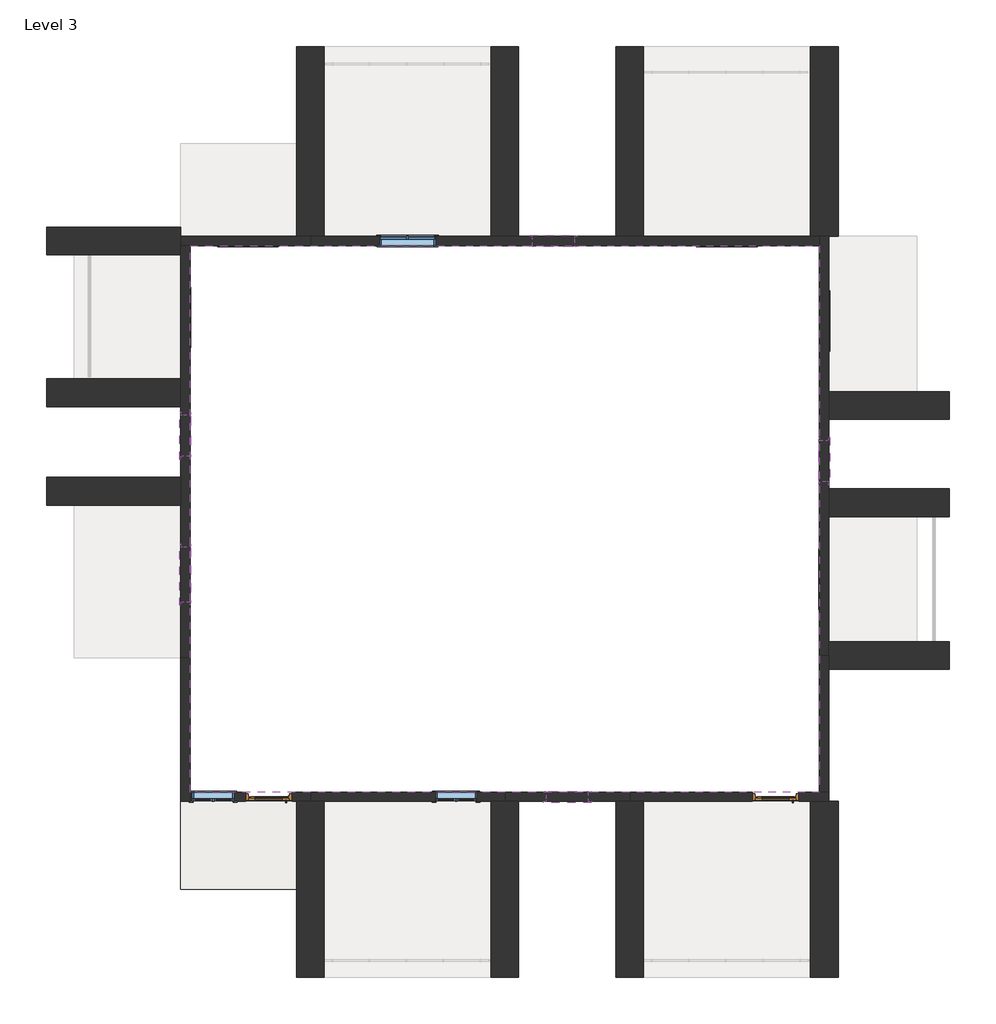
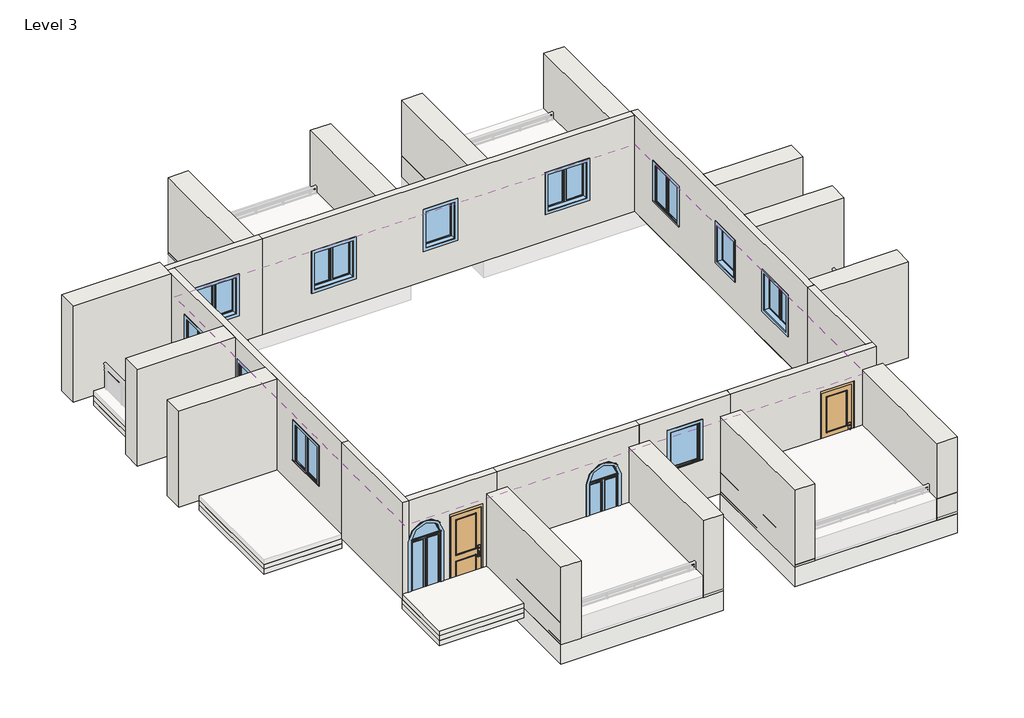
# One storey, part 1 of 2: 24 walls, 13 windows, 5 slabs, 2 doors, 1 covering.
"""IFC4 building model written with IfcOpenShell, lengths in millimetres."""

from ifc_helpers import new_model, si_unit, frame, origin, place, context, project, spatial, polyline, circle_curve, outline, extrude, faceted_brep, transform, mapped, element, save
from ifc_brep_helpers import plane_surface, revolved_surface, advanced_brep
from components import door_b6c2ee01, window_4e95f2a8, window_0862ab64, window_3a1167bf, window_8a4441b2

model = new_model("IFC4")

# Units and contexts
model_context = context("Model", 3, world=origin())
ifc_project = project(units=[si_unit("LENGTHUNIT", "METRE", prefix="MILLI")], contexts=[model_context])

# Site, building, storey
site = spatial("IfcSite", under=ifc_project)
building = spatial("IfcBuilding", under=site)
storey = spatial("IfcBuildingStorey", under=building, Name="Level 3", Elevation=6096.0)

# Covering
placement = place(None, origin())
element("IfcCovering", 1, ObjectType="2' x 4' ACT System", at=placement, inside=storey, context=model_context, shape_type="SweptSolid", body=[
    extrude(outline(polyline([(-12179.4937431, 6319.013611), (-9537.8937431, 6319.013611), (1638.1062569, 6319.013611), (1638.1062569, -2672.586389), (1638.1062569, -5669.786389), (-2527.4937431, -5669.786389), (-5270.6937431, -5669.786389), (-9537.8937431, -5669.786389), (-12179.4937431, -5669.786389), (-12179.4937431, -2723.386389), (-12179.4937431, 6319.013611)])), frame((0.0, 0.0, 8534.4), z_axis=(0.0, 0.0, 1.0), x_axis=(1.0, 0.0, 0.0)), (0.0, 0.0, 1.0), 57.15),
])

# Doors
door_shape = door_b6c2ee01(model_context)
element("IfcDoor", 2, ObjectType="Door-Exterior-Single-Two_Lite : 36\" x 94\"", at=placement, inside=storey, context=model_context, shape_type="MappedRepresentation", body=[
    mapped(door_shape, transform((-10452.2937431, -5765.036389, 6096.0), x_axis=(-1.0, 0.0, 0.0), y_axis=(0.0, -1.0, 0.0), z_axis=(0.0, 0.0, 1.0))),
])
element("IfcDoor", 3, ObjectType="Door-Exterior-Single-Two_Lite : 36\" x 94\"", at=placement, inside=storey, context=model_context, shape_type="MappedRepresentation", body=[
    mapped(door_shape, transform((672.9062569, -5765.036389, 6096.0), x_axis=(-1.0, 0.0, 0.0), y_axis=(0.0, -1.0, 0.0), z_axis=(0.0, 0.0, 1.0))),
])

# Slabs
element("IfcSlab", 4, ObjectType="Generic - 2' 2", at=placement, inside=storey, context=model_context, shape_type="SweptSolid", body=[
    extrude(outline(polyline([(-4965.8937431, -9733.786389), (-9842.6937431, -9733.786389), (-9842.6937431, -5872.986389), (-4965.8937431, -5872.986389), (-4965.8937431, -9733.786389)])), frame((0.0, 0.0, 5791.2), z_axis=(0.0, 0.0, 1.0), x_axis=(1.0, 0.0, 0.0)), (0.0, 0.0, 1.0), 609.6),
])
element("IfcSlab", 5, ObjectType="Generic - 2' 2", at=placement, inside=storey, context=model_context, shape_type="SweptSolid", body=[
    extrude(outline(polyline([(2044.5062569, -9733.786389), (-2832.2937431, -9733.786389), (-2832.2937431, -5872.986389), (2044.5062569, -5872.986389), (2044.5062569, -9733.786389)])), frame((0.0, 0.0, 5791.2), z_axis=(0.0, 0.0, 1.0), x_axis=(1.0, 0.0, 0.0)), (0.0, 0.0, 1.0), 609.6),
])
element("IfcSlab", 6, ObjectType="general 6\"", at=placement, inside=storey, context=model_context, shape_type="SweptSolid", body=[
    extrude(outline(polyline([(-14722.8064179, 6115.813611), (-12382.6937431, 6115.813611), (-12382.6937431, 3398.013611), (-14722.8064179, 3398.013611), (-14722.8064179, 6115.813611)])), frame((0.0, 0.0, 6096.0), z_axis=(0.0, 0.0, 1.0), x_axis=(1.0, 0.0, 0.0)), (0.0, 0.0, 1.0), 152.4),
    extrude(outline(polyline([(-14722.8064179, 629.413611), (-12382.6937431, 629.413611), (-12382.6937431, -2723.386389), (-14722.8064179, -2723.386389), (-14722.8064179, 629.413611)])), frame((0.0, 0.0, 6096.0), z_axis=(0.0, 0.0, 1.0), x_axis=(1.0, 0.0, 0.0)), (0.0, 0.0, 1.0), 152.4),
    extrude(outline(polyline([(-9842.6937431, -5872.986389), (-9842.6937431, -7803.386389), (-12382.6937431, -7803.386389), (-12382.6937431, -5872.986389), (-9842.6937431, -5872.986389)])), frame((0.0, 0.0, 6096.0), z_axis=(0.0, 0.0, 1.0), x_axis=(1.0, 0.0, 0.0)), (0.0, 0.0, 1.0), 152.4),
    extrude(outline(polyline([(3771.7062569, -2367.786389), (1841.3062569, -2367.786389), (1841.3062569, 426.213611), (3771.7062569, 426.213611), (3771.7062569, -2367.786389)])), frame((0.0, 0.0, 6096.0), z_axis=(0.0, 0.0, 1.0), x_axis=(1.0, 0.0, 0.0)), (0.0, 0.0, 1.0), 152.4),
    extrude(outline(polyline([(3771.7062569, 3118.613611), (1841.3062569, 3118.613611), (1841.3062569, 6522.213611), (3771.7062569, 6522.213611), (3771.7062569, 3118.613611)])), frame((0.0, 0.0, 6096.0), z_axis=(0.0, 0.0, 1.0), x_axis=(1.0, 0.0, 0.0)), (0.0, 0.0, 1.0), 152.4),
    extrude(outline(polyline([(-12382.6937431, 6522.213611), (-12382.6937431, 8557.6995084), (-9842.6937431, 8557.6995084), (-9842.6937431, 6522.213611), (-12382.6937431, 6522.213611)])), frame((0.0, 0.0, 6096.0), z_axis=(0.0, 0.0, 1.0), x_axis=(1.0, 0.0, 0.0)), (0.0, 0.0, 1.0), 152.4),
])
element("IfcSlab", 7, ObjectType="general 6\" 2", at=placement, inside=storey, context=model_context, shape_type="SweptSolid", body=[
    extrude(outline(polyline([(3771.7062569, -2367.786389), (1841.3062569, -2367.786389), (1841.3062569, 375.413611), (3771.7062569, 375.413611), (3771.7062569, -2367.786389)])), frame((0.0, 0.0, 6248.4), z_axis=(0.0, 0.0, 1.0), x_axis=(1.0, 0.0, 0.0)), (0.0, 0.0, 1.0), 152.4),
    extrude(outline(polyline([(3771.7062569, 3118.613611), (1841.3062569, 3118.613611), (1841.3062569, 6522.213611), (3771.7062569, 6522.213611), (3771.7062569, 3118.613611)])), frame((0.0, 0.0, 6248.4), z_axis=(0.0, 0.0, 1.0), x_axis=(1.0, 0.0, 0.0)), (0.0, 0.0, 1.0), 152.4),
    extrude(outline(polyline([(-12382.6937431, 6522.213611), (-12382.6937431, 8557.6995084), (-9842.6937431, 8557.6995084), (-9842.6937431, 6522.213611), (-12382.6937431, 6522.213611)])), frame((0.0, 0.0, 6248.4), z_axis=(0.0, 0.0, 1.0), x_axis=(1.0, 0.0, 0.0)), (0.0, 0.0, 1.0), 152.4),
    extrude(outline(polyline([(-14722.8064179, 6115.813611), (-12384.3500805, 6115.813611), (-12384.3500805, 3398.013611), (-14722.8064179, 3398.013611), (-14722.8064179, 6115.813611)])), frame((0.0, 0.0, 6248.4), z_axis=(0.0, 0.0, 1.0), x_axis=(1.0, 0.0, 0.0)), (0.0, 0.0, 1.0), 152.4),
    extrude(outline(polyline([(-14722.8064179, -2723.386389), (-14722.8064179, 629.413611), (-12382.6937431, 629.413611), (-12382.6937431, -2723.386389), (-14722.8064179, -2723.386389)])), frame((0.0, 0.0, 6248.4), z_axis=(0.0, 0.0, 1.0), x_axis=(1.0, 0.0, 0.0)), (0.0, 0.0, 1.0), 152.4),
    extrude(outline(polyline([(-9842.6937431, -5872.986389), (-9842.6937431, -7803.386389), (-12382.6937431, -7803.386389), (-12382.6937431, -5872.986389), (-9842.6937431, -5872.986389)])), frame((0.0, 0.0, 6248.4), z_axis=(0.0, 0.0, 1.0), x_axis=(1.0, 0.0, 0.0)), (0.0, 0.0, 1.0), 152.4),
])
element("IfcSlab", 8, ObjectType="general 6\" 3", at=placement, inside=storey, context=model_context, shape_type="SweptSolid", body=[
    extrude(outline(polyline([(-12382.6937431, -5872.986389), (-9842.6937431, -5872.986389), (-9842.6937431, -7803.386389), (-12382.6937431, -7803.386389), (-12382.6937431, -5872.986389)])), frame((0.0, 0.0, 6400.8), z_axis=(0.0, 0.0, 1.0), x_axis=(1.0, 0.0, 0.0)), (0.0, 0.0, 1.0), 152.4),
])

# Walls
element("IfcWall", 9, ObjectType="Generic - 8\"", at=placement, inside=storey, context=model_context, shape_type="Brep", body=[
    faceted_brep([(-12382.6937431, 6319.013611, 6400.8), (-12179.4937431, 6319.013611, 6400.8), (-9537.8937431, 6319.013611, 6400.8), (-9537.8937431, 6319.013611, 9448.8), (-12179.4937431, 6319.013611, 9448.8), (-12382.6937431, 6319.013611, 9448.8), (-10299.8937431, 6319.013611, 8534.4), (-10299.8937431, 6319.013611, 7315.2), (-11519.0937431, 6319.013611, 7315.2), (-11519.0937431, 6319.013611, 8534.4), (-12382.6937431, 6522.213611, 6400.8), (-12382.6937431, 6522.213611, 9448.8), (-9537.8937431, 6522.213611, 9448.8), (-9537.8937431, 6522.213611, 6400.8), (-9842.6937431, 6522.213611, 6400.8), (-10299.8937431, 6522.213611, 8534.4), (-11519.0937431, 6522.213611, 8534.4), (-11519.0937431, 6522.213611, 7315.2), (-10299.8937431, 6522.213611, 7315.2)], [[[0, 1, 2, 3, 4, 5], [6, 7, 8, 9]], [[10, 11, 12, 13, 14], [15, 16, 17, 18]], [[2, 1, 0, 10, 14, 13]], [[5, 4, 3, 12, 11]], [[0, 5, 11, 10]], [[7, 6, 15, 18]], [[8, 7, 18, 17]], [[9, 8, 17, 16]], [[6, 9, 16, 15]], [[2, 13, 12, 3]]]),
])
element("IfcWall", 10, ObjectType="Generic - 8\"", at=placement, inside=storey, context=model_context, shape_type="Brep", body=[
    faceted_brep([(-12179.4937431, -5872.986389, 6400.8), (-12179.4937431, -5669.786389, 6400.8), (-12179.4937431, -2723.386389, 6400.8), (-12179.4937431, -2723.386389, 9448.8), (-12179.4937431, -5669.786389, 9448.8), (-12179.4937431, -5872.986389, 9448.8), (-12382.6937431, -5872.986389, 6400.8), (-12382.6937431, -5872.986389, 9448.8), (-12382.6937431, -2723.386389, 9448.8), (-12382.6937431, -2723.386389, 6400.8)], [[[0, 1, 2, 3, 4, 5]], [[6, 7, 8, 9]], [[2, 1, 0, 6, 9]], [[3, 2, 9, 8]], [[5, 4, 3, 8, 7]], [[0, 5, 7, 6]]]),
])
element("IfcWall", 11, ObjectType="Generic - 8\"", at=placement, inside=storey, context=model_context, shape_type="Brep", body=[
    faceted_brep([(-2527.4937431, -5669.786389, 9448.8), (1638.1062569, -5669.786389, 9448.8), (1841.3062569, -5669.786389, 9448.8), (1841.3062569, -5669.786389, 6400.8), (1638.1062569, -5669.786389, 6400.8), (1180.9062569, -5669.786389, 6400.8), (1180.9062569, -5669.786389, 8585.2), (164.9062569, -5669.786389, 8585.2), (164.9062569, -5669.786389, 6400.8), (-2527.4937431, -5669.786389, 6400.8), (1841.3062569, -5872.986389, 9448.8), (-2527.4937431, -5872.986389, 9448.8), (-2527.4937431, -5872.986389, 6400.8), (-2222.6937431, -5872.986389, 6400.8), (164.9062569, -5872.986389, 6400.8), (164.9062569, -5872.986389, 8585.2), (1180.9062569, -5872.986389, 8585.2), (1180.9062569, -5872.986389, 6400.8), (1434.9062569, -5872.986389, 6400.8), (1841.3062569, -5872.986389, 6400.8)], [[[0, 1, 2, 3, 4, 5, 6, 7, 8, 9]], [[10, 11, 12, 13, 14, 15, 16, 17, 18, 19]], [[3, 19, 18, 17, 5, 4]], [[12, 9, 8, 14, 13]], [[2, 1, 0, 11, 10]], [[2, 10, 19, 3]], [[7, 15, 14, 8]], [[15, 7, 6, 16]], [[16, 6, 5, 17]], [[9, 12, 11, 0]]]),
])
element("IfcWall", 12, ObjectType="Generic - 8\"", at=placement, inside=storey, context=model_context, shape_type="Brep", body=[
    faceted_brep([(1638.1062569, 6522.213611, 9448.8), (1638.1062569, 6522.213611, 6400.8), (1638.1062569, 6319.013611, 6400.8), (1638.1062569, -2672.586389, 6400.8), (1638.1062569, -2672.586389, 9448.8), (1638.1062569, 6319.013611, 9448.8), (1638.1062569, 1137.413611, 8605.6747769), (1638.1062569, 1137.413611, 7386.4747769), (1638.1062569, 2051.813611, 7386.4747769), (1638.1062569, 2051.813611, 8605.6747769), (1638.1062569, -1605.786389, 8545.5712595), (1638.1062569, -1605.786389, 7326.3712595), (1638.1062569, -386.586389, 7326.3712595), (1638.1062569, -386.586389, 8545.5712595), (1638.1062569, 4058.413611, 8545.5712595), (1638.1062569, 4058.413611, 7326.3712595), (1638.1062569, 5277.613611, 7326.3712595), (1638.1062569, 5277.613611, 8545.5712595), (1841.3062569, 6522.213611, 6400.8), (1841.3062569, 6522.213611, 9448.8), (1841.3062569, 3118.613611, 9448.8), (1841.3062569, 2509.013611, 9448.8), (1841.3062569, 985.013611, 9448.8), (1841.3062569, 375.413611, 9448.8), (1841.3062569, -2367.786389, 9448.8), (1841.3062569, -2672.586389, 9448.8), (1841.3062569, -2672.586389, 6400.8), (1841.3062569, -2367.786389, 6400.8), (1841.3062569, 375.413611, 6400.8), (1841.3062569, 985.013611, 6400.8), (1841.3062569, 2509.013611, 6400.8), (1841.3062569, 3118.613611, 6400.8), (1841.3062569, 1137.413611, 8605.6747769), (1841.3062569, 2051.813611, 8605.6747769), (1841.3062569, 2051.813611, 7386.4747769), (1841.3062569, 1137.413611, 7386.4747769), (1841.3062569, -1605.786389, 8545.5712595), (1841.3062569, -386.586389, 8545.5712595), (1841.3062569, -386.586389, 7326.3712595), (1841.3062569, -1605.786389, 7326.3712595), (1841.3062569, 4058.413611, 8545.5712595), (1841.3062569, 5277.613611, 8545.5712595), (1841.3062569, 5277.613611, 7326.3712595), (1841.3062569, 4058.413611, 7326.3712595)], [[[0, 1, 2, 3, 4, 5], [6, 7, 8, 9], [10, 11, 12, 13], [14, 15, 16, 17]], [[18, 19, 20, 21, 22, 23, 24, 25, 26, 27, 28, 29, 30, 31], [32, 33, 34, 35], [36, 37, 38, 39], [40, 41, 42, 43]], [[3, 2, 1, 18, 31, 30, 29, 28, 27, 26]], [[4, 3, 26, 25]], [[0, 5, 4, 25, 24, 23, 22, 21, 20, 19]], [[0, 19, 18, 1]], [[7, 6, 32, 35]], [[8, 7, 35, 34]], [[9, 8, 34, 33]], [[6, 9, 33, 32]], [[11, 10, 36, 39]], [[12, 11, 39, 38]], [[13, 12, 38, 37]], [[10, 13, 37, 36]], [[15, 14, 40, 43]], [[16, 15, 43, 42]], [[17, 16, 42, 41]], [[14, 17, 41, 40]]]),
])
element("IfcWall", 13, ObjectType="Generic - 8\"", at=placement, inside=storey, context=model_context, shape_type="Brep", body=[
    faceted_brep([(-12179.4937431, -2723.386389, 6400.8), (-12179.4937431, 6319.013611, 6400.8), (-12179.4937431, 6319.013611, 9448.8), (-12179.4937431, -2723.386389, 9448.8), (-12179.4937431, 2610.613611, 8771.7149116), (-12179.4937431, 2610.613611, 7552.5149116), (-12179.4937431, 1696.213611, 7552.5149116), (-12179.4937431, 1696.213611, 8771.7149116), (-12179.4937431, -284.986389, 8594.8059909), (-12179.4937431, -284.986389, 7375.6059909), (-12179.4937431, -1504.186389, 7375.6059909), (-12179.4937431, -1504.186389, 8594.8059909), (-12179.4937431, 5353.813611, 8521.1335827), (-12179.4937431, 5353.813611, 7301.9335827), (-12179.4937431, 4134.613611, 7301.9335827), (-12179.4937431, 4134.613611, 8521.1335827), (-12382.6937431, -2723.386389, 6400.8), (-12382.6937431, -2723.386389, 9448.8), (-12382.6937431, 629.413611, 9448.8), (-12382.6937431, 1239.013611, 9448.8), (-12382.6937431, 2788.413611, 9448.8), (-12382.6937431, 3398.013611, 9448.8), (-12382.6937431, 6115.813611, 9448.8), (-12382.6937431, 6319.013611, 9448.8), (-12382.6937431, 6319.013611, 6400.8), (-12382.6937431, 6115.813611, 6400.8), (-12382.6937431, 3398.013611, 6400.8), (-12382.6937431, 2788.413611, 6400.8), (-12382.6937431, 1239.013611, 6400.8), (-12382.6937431, 629.413611, 6400.8), (-12382.6937431, 2610.613611, 8771.7149116), (-12382.6937431, 1696.213611, 8771.7149116), (-12382.6937431, 1696.213611, 7552.5149116), (-12382.6937431, 2610.613611, 7552.5149116), (-12382.6937431, -284.986389, 8594.8059909), (-12382.6937431, -1504.186389, 8594.8059909), (-12382.6937431, -1504.186389, 7375.6059909), (-12382.6937431, -284.986389, 7375.6059909), (-12382.6937431, 5353.813611, 8521.1335827), (-12382.6937431, 4134.613611, 8521.1335827), (-12382.6937431, 4134.613611, 7301.9335827), (-12382.6937431, 5353.813611, 7301.9335827)], [[[0, 1, 2, 3], [4, 5, 6, 7], [8, 9, 10, 11], [12, 13, 14, 15]], [[16, 17, 18, 19, 20, 21, 22, 23, 24, 25, 26, 27, 28, 29], [30, 31, 32, 33], [34, 35, 36, 37], [38, 39, 40, 41]], [[1, 0, 16, 29, 28, 27, 26, 25, 24]], [[3, 2, 23, 22, 21, 20, 19, 18, 17]], [[0, 3, 17, 16]], [[2, 1, 24, 23]], [[5, 4, 30, 33]], [[6, 5, 33, 32]], [[7, 6, 32, 31]], [[4, 7, 31, 30]], [[9, 8, 34, 37]], [[10, 9, 37, 36]], [[11, 10, 36, 35]], [[8, 11, 35, 34]], [[13, 12, 38, 41]], [[14, 13, 41, 40]], [[15, 14, 40, 39]], [[12, 15, 39, 38]]]),
])
element("IfcWall", 14, ObjectType="Generic - 8\"", at=placement, inside=storey, context=model_context, shape_type="AdvancedBrep", body=[
    advanced_brep(
    [(-12179.4937431, -5669.786389, 9448.8), (-9537.8937431, -5669.786389, 9448.8), (-9537.8937431, -5669.786389, 6400.8), (-9944.2937431, -5669.786389, 6400.8), (-9944.2937431, -5669.786389, 8585.2), (-10960.2937431, -5669.786389, 8585.2), (-10960.2937431, -5669.786389, 6400.8), (-11214.2937431, -5669.786389, 6400.8), (-11214.2937431, -5669.786389, 8139.597687), (-12128.6937431, -5669.786389, 8139.597687), (-12128.6937431, -5669.786389, 6400.8), (-12179.4937431, -5669.786389, 6400.8), (-9537.8937431, -5872.986389, 9448.8), (-12179.4937431, -5872.986389, 9448.8), (-12179.4937431, -5872.986389, 6400.8), (-12128.6937431, -5872.986389, 6400.8), (-12128.6937431, -5872.986389, 8139.597687), (-11214.2937431, -5872.986389, 8139.597687), (-11214.2937431, -5872.986389, 6400.8), (-10960.2937431, -5872.986389, 6400.8), (-10960.2937431, -5872.986389, 8585.2), (-9944.2937431, -5872.986389, 8585.2), (-9944.2937431, -5872.986389, 6400.8), (-9842.6937431, -5872.986389, 6400.8), (-9537.8937431, -5872.986389, 6400.8)],
    [
        (0, 1),
        (1, 2),
        (2, 3),
        (3, 4),
        (4, 5),
        (5, 6),
        (6, 7),
        (7, 8),
        (8, 9, circle_curve(frame((-11671.4937431, -5669.786389, 8139.597687), z_axis=(0.0, -1.0, 0.0), x_axis=(-1.0, 0.0, 0.0)), 457.2)),
        (9, 10),
        (10, 11),
        (11, 0),
        (12, 13),
        (13, 14),
        (14, 15),
        (15, 16),
        (16, 17, circle_curve(frame((-11671.4937431, -5872.986389, 8139.597687), z_axis=(0.0, 1.0, 0.0), x_axis=(-1.0, 0.0, 0.0)), 457.2)),
        (17, 18),
        (18, 19),
        (19, 20),
        (20, 21),
        (21, 22),
        (22, 23),
        (23, 24),
        (24, 12),
        (14, 11),
        (10, 15),
        (2, 24),
        (22, 3),
        (6, 19),
        (18, 7),
        (0, 13),
        (12, 1),
        (5, 20),
        (4, 21),
        (9, 16),
        (17, 8),
    ],
    [
        plane_surface(frame((1423.3958892, -5669.786389, 6400.8), z_axis=(0.0, 1.0, 0.0), x_axis=(-1.0, 0.0, 0.0))),
        plane_surface(frame((1423.3958892, -5872.986389, 6400.8), z_axis=(0.0, -1.0, 0.0), x_axis=(1.0, 0.0, 0.0))),
        plane_surface(frame((-9537.8937431, -5669.786389, 6400.8), z_axis=(0.0, 0.0, -1.0), x_axis=(0.0, -1.0, 0.0))),
        plane_surface(frame((-12281.0937431, -5669.786389, 9448.8), z_axis=(0.0, 0.0, 1.0), x_axis=(0.0, -1.0, 0.0))),
        plane_surface(frame((-12179.4937431, 6416.9740134, 6400.8), z_axis=(-1.0, 0.0, 0.0), x_axis=(0.0, 1.0, 0.0))),
        plane_surface(frame((-9537.8937431, -5669.786389, 9448.8), z_axis=(1.0, 0.0, 0.0), x_axis=(0.0, -1.0, 0.0))),
        plane_surface(frame((-10960.2937431, -4145.786389, 6096.0), z_axis=(1.0, 0.0, 0.0), x_axis=(0.0, -1.0, 0.0))),
        plane_surface(frame((-10960.2937431, -4145.786389, 8585.2), z_axis=(0.0, 0.0, -1.0), x_axis=(0.0, -1.0, 0.0))),
        plane_surface(frame((-9944.2937431, -4145.786389, 8585.2), z_axis=(-1.0, 0.0, 0.0), x_axis=(0.0, -1.0, 0.0))),
        plane_surface(frame((-12128.6937431, -7193.786389, 8139.597687), z_axis=(1.0, 0.0, 0.0), x_axis=(0.0, 1.0, 0.0))),
        plane_surface(frame((-11214.2937431, -7193.786389, 6291.747687), z_axis=(-1.0, 0.0, 0.0), x_axis=(0.0, 1.0, 0.0))),
        revolved_surface(polyline([(-12128.6937431, -5872.986389, 8139.597687), (-12128.6937431, -5669.786389, 8139.597687)]), (-11671.4937431, -4145.786389, 8139.597687), (0.0, -1.0, 0.0)),
    ],
    [
        (0, [[1, 2, 3, 4, 5, 6, 7, 8, 9, 10, 11, 12]]),
        (1, [[13, 14, 15, 16, 17, 18, 19, 20, 21, 22, 23, 24, 25]]),
        (2, [[26, -11, 27, -15]]),
        (2, [[28, -24, -23, 29, -3]]),
        (2, [[30, -19, 31, -7]]),
        (3, [[-1, 32, -13, 33]]),
        (4, [[-12, -26, -14, -32]]),
        (5, [[-33, -25, -28, -2]]),
        (6, [[34, -20, -30, -6]]),
        (7, [[-34, -5, 35, -21]]),
        (8, [[-35, -4, -29, -22]]),
        (9, [[36, -16, -27, -10]]),
        (10, [[37, -8, -31, -18]]),
        (11, [[-36, -9, -37, -17]]),
    ],
),
])
element("IfcWall", 15, ObjectType="Generic - 8\"", at=placement, inside=storey, context=model_context, shape_type="Brep", body=[
    faceted_brep([(1638.1062569, -2672.586389, 6400.8), (1638.1062569, -5669.786389, 6400.8), (1638.1062569, -5669.786389, 9448.8), (1638.1062569, -2672.586389, 9448.8), (1841.3062569, -2672.586389, 6400.8), (1841.3062569, -2672.586389, 9448.8), (1841.3062569, -2977.386389, 9448.8), (1841.3062569, -5669.786389, 9448.8), (1841.3062569, -5669.786389, 6400.8), (1841.3062569, -2977.386389, 6400.8)], [[[0, 1, 2, 3]], [[4, 5, 6, 7, 8, 9]], [[1, 0, 4, 9, 8]], [[3, 2, 7, 6, 5]], [[0, 3, 5, 4]], [[1, 8, 7, 2]]]),
])
element("IfcWall", 16, ObjectType="Generic - 8\"", at=placement, inside=storey, context=model_context, shape_type="Brep", body=[
    faceted_brep([(-9537.8937431, 6319.013611, 9448.8), (-9537.8937431, 6319.013611, 6400.8), (1638.1062569, 6319.013611, 6400.8), (1638.1062569, 6319.013611, 9448.8), (-3746.6937431, 6319.013611, 8632.3983257), (-3746.6937431, 6319.013611, 7413.1983257), (-4661.0937431, 6319.013611, 7413.1983257), (-4661.0937431, 6319.013611, 8632.3983257), (-6794.6937431, 6319.013611, 8481.182989), (-6794.6937431, 6319.013611, 7261.982989), (-8013.8937431, 6319.013611, 7261.982989), (-8013.8937431, 6319.013611, 8481.182989), (215.7062569, 6319.013611, 8518.4159819), (215.7062569, 6319.013611, 7299.2159819), (-1003.4937431, 6319.013611, 7299.2159819), (-1003.4937431, 6319.013611, 8518.4159819), (-9537.8937431, 6522.213611, 6400.8), (-9537.8937431, 6522.213611, 9448.8), (1638.1062569, 6522.213611, 9448.8), (1638.1062569, 6522.213611, 6400.8), (1434.9062569, 6522.213611, 6400.8), (-2222.6937431, 6522.213611, 6400.8), (-2832.2937431, 6522.213611, 6400.8), (-4965.8937431, 6522.213611, 6400.8), (-5575.4937431, 6522.213611, 6400.8), (-9233.0937431, 6522.213611, 6400.8), (-3746.6937431, 6522.213611, 8632.3983257), (-4661.0937431, 6522.213611, 8632.3983257), (-4661.0937431, 6522.213611, 7413.1983257), (-3746.6937431, 6522.213611, 7413.1983257), (-6794.6937431, 6522.213611, 8481.182989), (-8013.8937431, 6522.213611, 8481.182989), (-8013.8937431, 6522.213611, 7261.982989), (-6794.6937431, 6522.213611, 7261.982989), (215.7062569, 6522.213611, 8518.4159819), (-1003.4937431, 6522.213611, 8518.4159819), (-1003.4937431, 6522.213611, 7299.2159819), (215.7062569, 6522.213611, 7299.2159819)], [[[0, 1, 2, 3], [4, 5, 6, 7], [8, 9, 10, 11], [12, 13, 14, 15]], [[16, 17, 18, 19, 20, 21, 22, 23, 24, 25], [26, 27, 28, 29], [30, 31, 32, 33], [34, 35, 36, 37]], [[2, 1, 16, 25, 24, 23, 22, 21, 20, 19]], [[0, 3, 18, 17]], [[2, 19, 18, 3]], [[5, 4, 26, 29]], [[6, 5, 29, 28]], [[7, 6, 28, 27]], [[4, 7, 27, 26]], [[9, 8, 30, 33]], [[10, 9, 33, 32]], [[11, 10, 32, 31]], [[8, 11, 31, 30]], [[13, 12, 34, 37]], [[14, 13, 37, 36]], [[15, 14, 36, 35]], [[12, 15, 35, 34]], [[0, 17, 16, 1]]]),
])
element("IfcWall", 17, ObjectType="Generic - 8\"", at=placement, inside=storey, context=model_context, shape_type="Brep", body=[
    faceted_brep([(-2527.4937431, -5669.786389, 9448.8), (-2527.4937431, -5669.786389, 6400.8), (-5270.6937431, -5669.786389, 6400.8), (-5270.6937431, -5669.786389, 9448.8), (-4356.2937431, -5669.786389, 8895.074951), (-4356.2937431, -5669.786389, 7675.874951), (-3441.8937431, -5669.786389, 7675.874951), (-3441.8937431, -5669.786389, 8895.074951), (-2527.4937431, -5872.986389, 6400.8), (-2527.4937431, -5872.986389, 9448.8), (-5270.6937431, -5872.986389, 9448.8), (-5270.6937431, -5872.986389, 6400.8), (-4965.8937431, -5872.986389, 6400.8), (-2832.2937431, -5872.986389, 6400.8), (-4356.2937431, -5872.986389, 8895.074951), (-3441.8937431, -5872.986389, 8895.074951), (-3441.8937431, -5872.986389, 7675.874951), (-4356.2937431, -5872.986389, 7675.874951)], [[[0, 1, 2, 3], [4, 5, 6, 7]], [[8, 9, 10, 11, 12, 13], [14, 15, 16, 17]], [[2, 1, 8, 13, 12, 11]], [[0, 3, 10, 9]], [[5, 4, 14, 17]], [[6, 5, 17, 16]], [[7, 6, 16, 15]], [[4, 7, 15, 14]], [[0, 9, 8, 1]], [[2, 11, 10, 3]]]),
])
element("IfcWall", 18, ObjectType="Generic - 8\"", at=placement, inside=storey, context=model_context, shape_type="AdvancedBrep", body=[
    advanced_brep(
    [(-9537.8937431, -5669.786389, 9448.8), (-5270.6937431, -5669.786389, 9448.8), (-5270.6937431, -5669.786389, 6400.8), (-5880.2937431, -5669.786389, 6400.8), (-5880.2937431, -5669.786389, 8096.25), (-6794.6937431, -5669.786389, 8096.25), (-6794.6937431, -5669.786389, 6400.8), (-9537.8937431, -5669.786389, 6400.8), (-5270.6937431, -5872.986389, 9448.8), (-9537.8937431, -5872.986389, 9448.8), (-9537.8937431, -5872.986389, 6400.8), (-9233.0937431, -5872.986389, 6400.8), (-6794.6937431, -5872.986389, 6400.8), (-6794.6937431, -5872.986389, 8096.25), (-5880.2937431, -5872.986389, 8096.25), (-5880.2937431, -5872.986389, 6400.8), (-5575.4937431, -5872.986389, 6400.8), (-5270.6937431, -5872.986389, 6400.8)],
    [
        (0, 1),
        (1, 2),
        (2, 3),
        (3, 4),
        (4, 5, circle_curve(frame((-6337.4937431, -5669.786389, 8096.25), z_axis=(0.0, -1.0, 0.0), x_axis=(-1.0, 0.0, 0.0)), 457.2)),
        (5, 6),
        (6, 7),
        (7, 0),
        (8, 9),
        (9, 10),
        (10, 11),
        (11, 12),
        (12, 13),
        (13, 14, circle_curve(frame((-6337.4937431, -5872.986389, 8096.25), z_axis=(0.0, 1.0, 0.0), x_axis=(-1.0, 0.0, 0.0)), 457.2)),
        (14, 15),
        (15, 16),
        (16, 17),
        (17, 8),
        (10, 7),
        (6, 12),
        (2, 17),
        (15, 3),
        (0, 9),
        (8, 1),
        (5, 13),
        (14, 4),
    ],
    [
        plane_surface(frame((1423.3958892, -5669.786389, 6400.8), z_axis=(0.0, 1.0, 0.0), x_axis=(-1.0, 0.0, 0.0))),
        plane_surface(frame((1423.3958892, -5872.986389, 6400.8), z_axis=(0.0, -1.0, 0.0), x_axis=(1.0, 0.0, 0.0))),
        plane_surface(frame((-5270.6937431, -5669.786389, 6400.8), z_axis=(0.0, 0.0, -1.0), x_axis=(0.0, -1.0, 0.0))),
        plane_surface(frame((-9537.8937431, -5669.786389, 9448.8), z_axis=(0.0, 0.0, 1.0), x_axis=(0.0, -1.0, 0.0))),
        plane_surface(frame((-6794.6937431, -7193.786389, 8096.25), z_axis=(1.0, 0.0, 0.0), x_axis=(0.0, 1.0, 0.0))),
        plane_surface(frame((-5880.2937431, -7193.786389, 6248.4), z_axis=(-1.0, 0.0, 0.0), x_axis=(0.0, 1.0, 0.0))),
        revolved_surface(polyline([(-6794.6937431, -5872.986389, 8096.25), (-6794.6937431, -5669.786389, 8096.25)]), (-6337.4937431, -4145.786389, 8096.25), (0.0, -1.0, 0.0)),
        plane_surface(frame((-5270.6937431, -5669.786389, 9448.8), z_axis=(1.0, 0.0, 0.0), x_axis=(0.0, -1.0, 0.0))),
        plane_surface(frame((-9537.8937431, -5669.786389, 6400.8), z_axis=(-1.0, 0.0, 0.0), x_axis=(0.0, -1.0, 0.0))),
    ],
    [
        (0, [[1, 2, 3, 4, 5, 6, 7, 8]]),
        (1, [[9, 10, 11, 12, 13, 14, 15, 16, 17, 18]]),
        (2, [[19, -7, 20, -12, -11]]),
        (2, [[21, -17, -16, 22, -3]]),
        (3, [[-1, 23, -9, 24]]),
        (4, [[25, -13, -20, -6]]),
        (5, [[26, -4, -22, -15]]),
        (6, [[-25, -5, -26, -14]]),
        (7, [[-24, -18, -21, -2]]),
        (8, [[-19, -10, -23, -8]]),
    ],
),
])
element("IfcWall", 19, ObjectType="Generic -2' 2", at=placement, inside=storey, context=model_context, shape_type="Brep", body=[
    faceted_brep([(-12382.6937431, 6725.413611, 6400.8), (-15329.0937431, 6725.413611, 6400.8), (-15329.0937431, 6725.413611, 9448.8), (-12382.6937431, 6725.413611, 9448.8), (-12382.6937431, 6115.813611, 6400.8), (-12382.6937431, 6115.813611, 9448.8), (-15329.0937431, 6115.813611, 9448.8), (-15329.0937431, 6115.813611, 6400.8), (-12382.6937431, 6522.213611, 6400.8), (-12382.6937431, 6319.013611, 6400.8), (-12382.6937431, 6319.013611, 9448.8), (-12382.6937431, 6522.213611, 9448.8)], [[[0, 1, 2, 3]], [[4, 5, 6, 7]], [[1, 0, 8, 9, 4, 7]], [[2, 1, 7, 6]], [[3, 2, 6, 5, 10, 11]], [[0, 3, 11, 10, 5, 4, 9, 8]]]),
])
element("IfcWall", 20, ObjectType="Generic -2' 2", at=placement, inside=storey, context=model_context, shape_type="SweptSolid", body=[
    extrude(outline(polyline([(-15329.0937431, 3398.013611), (-12382.6937431, 3398.013611), (-12382.6937431, 2788.413611), (-15329.0937431, 2788.413611), (-15329.0937431, 3398.013611)])), frame((0.0, 0.0, 6400.8), z_axis=(0.0, 0.0, 1.0), x_axis=(1.0, 0.0, 0.0)), (0.0, 0.0, 1.0), 3048.0),
])
element("IfcWall", 21, ObjectType="Generic -2' 2", at=placement, inside=storey, context=model_context, shape_type="SweptSolid", body=[
    extrude(outline(polyline([(-15329.0937431, 1239.013611), (-12382.6937431, 1239.013611), (-12382.6937431, 629.413611), (-15329.0937431, 629.413611), (-15329.0937431, 1239.013611)])), frame((0.0, 0.0, 6400.8), z_axis=(0.0, 0.0, 1.0), x_axis=(1.0, 0.0, 0.0)), (0.0, 0.0, 1.0), 3048.0),
])
element("IfcWall", 22, ObjectType="Generic -2' 2", at=placement, inside=storey, context=model_context, shape_type="Brep", body=[
    faceted_brep([(1841.3062569, -2977.386389, 6400.8), (4482.9062569, -2977.386389, 6400.8), (4482.9062569, -2977.386389, 9448.8), (1841.3062569, -2977.386389, 9448.8), (1841.3062569, -2367.786389, 6400.8), (1841.3062569, -2367.786389, 9448.8), (4482.9062569, -2367.786389, 9448.8), (4482.9062569, -2367.786389, 6400.8), (1841.3062569, -2672.586389, 6400.8), (1841.3062569, -2672.586389, 9448.8)], [[[0, 1, 2, 3]], [[4, 5, 6, 7]], [[1, 0, 8, 4, 7]], [[2, 1, 7, 6]], [[3, 2, 6, 5, 9]], [[0, 3, 9, 5, 4, 8]]]),
])
element("IfcWall", 23, ObjectType="Generic -2' 2", at=placement, inside=storey, context=model_context, shape_type="SweptSolid", body=[
    extrude(outline(polyline([(4482.9062569, 375.413611), (1841.3062569, 375.413611), (1841.3062569, 985.013611), (4482.9062569, 985.013611), (4482.9062569, 375.413611)])), frame((0.0, 0.0, 6400.8), z_axis=(0.0, 0.0, 1.0), x_axis=(1.0, 0.0, 0.0)), (0.0, 0.0, 1.0), 3048.0),
])
element("IfcWall", 24, ObjectType="Generic -2' 2", at=placement, inside=storey, context=model_context, shape_type="SweptSolid", body=[
    extrude(outline(polyline([(4482.9062569, 2509.013611), (1841.3062569, 2509.013611), (1841.3062569, 3118.613611), (4482.9062569, 3118.613611), (4482.9062569, 2509.013611)])), frame((0.0, 0.0, 6400.8), z_axis=(0.0, 0.0, 1.0), x_axis=(1.0, 0.0, 0.0)), (0.0, 0.0, 1.0), 3048.0),
])
element("IfcWall", 25, ObjectType="Generic -2' 3 red", at=placement, inside=storey, context=model_context, shape_type="Brep", body=[
    faceted_brep([(1434.9062569, -5872.986389, 6400.8), (1434.9062569, -9733.786389, 6400.8), (1434.9062569, -9733.786389, 8839.2), (1434.9062569, -5872.986389, 8839.2), (2044.5062569, -5872.986389, 6400.8), (2044.5062569, -5872.986389, 8839.2), (2044.5062569, -9733.786389, 8839.2), (2044.5062569, -9733.786389, 6400.8), (1841.3062569, -5872.986389, 6400.8)], [[[0, 1, 2, 3]], [[4, 5, 6, 7]], [[1, 0, 8, 4, 7]], [[2, 1, 7, 6]], [[3, 2, 6, 5]], [[0, 3, 5, 4, 8]]]),
])
element("IfcWall", 26, ObjectType="Generic -2' 3 red", at=placement, inside=storey, context=model_context, shape_type="Brep", body=[
    faceted_brep([(-2832.2937431, -5872.986389, 6400.8), (-2832.2937431, -9733.786389, 6400.8), (-2832.2937431, -9733.786389, 8846.8571637), (-2832.2937431, -5872.986389, 8846.8571637), (-2222.6937431, -5872.986389, 6400.8), (-2222.6937431, -5872.986389, 8846.8571637), (-2222.6937431, -9733.786389, 8846.8571637), (-2222.6937431, -9733.786389, 6400.8), (-2527.4937431, -5872.986389, 6400.8)], [[[0, 1, 2, 3]], [[4, 5, 6, 7]], [[1, 0, 8, 4, 7]], [[2, 1, 7, 6]], [[3, 2, 6, 5]], [[0, 3, 5, 4, 8]]]),
])
element("IfcWall", 27, ObjectType="Generic -2' 3 red", at=placement, inside=storey, context=model_context, shape_type="Brep", body=[
    faceted_brep([(-5575.4937431, -5872.986389, 6400.8), (-5575.4937431, -9733.786389, 6400.8), (-5575.4937431, -9733.786389, 8839.2), (-5575.4937431, -5872.986389, 8839.2), (-4965.8937431, -5872.986389, 6400.8), (-4965.8937431, -5872.986389, 8839.2), (-4965.8937431, -9733.786389, 8839.2), (-4965.8937431, -9733.786389, 6400.8), (-5270.6937431, -5872.986389, 6400.8)], [[[0, 1, 2, 3]], [[4, 5, 6, 7]], [[1, 0, 8, 4, 7]], [[2, 1, 7, 6]], [[3, 2, 6, 5]], [[0, 3, 5, 4, 8]]]),
])
element("IfcWall", 28, ObjectType="Generic -2' 3 red", at=placement, inside=storey, context=model_context, shape_type="Brep", body=[
    faceted_brep([(-9842.6937431, -5872.986389, 6400.8), (-9842.6937431, -9733.786389, 6400.8), (-9842.6937431, -9733.786389, 8859.7612992), (-9842.6937431, -5872.986389, 8859.7612992), (-9233.0937431, -5872.986389, 6400.8), (-9233.0937431, -5872.986389, 8859.7612992), (-9233.0937431, -9733.786389, 8859.7612992), (-9233.0937431, -9733.786389, 6400.8), (-9537.8937431, -5872.986389, 6400.8)], [[[0, 1, 2, 3]], [[4, 5, 6, 7]], [[1, 0, 8, 4, 7]], [[2, 1, 7, 6]], [[3, 2, 6, 5]], [[0, 3, 5, 4, 8]]]),
])
element("IfcWall", 29, ObjectType="Generic -2' 3 red", at=placement, inside=storey, context=model_context, shape_type="Brep", body=[
    faceted_brep([(-9233.0937431, 6522.213611, 6400.8), (-9233.0937431, 10687.813611, 6400.8), (-9233.0937431, 10687.813611, 8839.2), (-9233.0937431, 6522.213611, 8839.2), (-9842.6937431, 6522.213611, 6400.8), (-9842.6937431, 6522.213611, 8839.2), (-9842.6937431, 10687.813611, 8839.2), (-9842.6937431, 10687.813611, 6400.8), (-9537.8937431, 6522.213611, 6400.8)], [[[0, 1, 2, 3]], [[4, 5, 6, 7]], [[1, 0, 8, 4, 7]], [[2, 1, 7, 6]], [[3, 2, 6, 5]], [[0, 3, 5, 4, 8]]]),
])
element("IfcWall", 30, ObjectType="Generic -2' 3 red", at=placement, inside=storey, context=model_context, shape_type="SweptSolid", body=[
    extrude(outline(polyline([(-4965.8937431, 10687.813611), (-4965.8937431, 6522.213611), (-5575.4937431, 6522.213611), (-5575.4937431, 10687.813611), (-4965.8937431, 10687.813611)])), frame((0.0, 0.0, 6400.8), z_axis=(0.0, 0.0, 1.0), x_axis=(1.0, 0.0, 0.0)), (0.0, 0.0, 1.0), 2443.0998934),
])
element("IfcWall", 31, ObjectType="Generic -2' 3 red", at=placement, inside=storey, context=model_context, shape_type="SweptSolid", body=[
    extrude(outline(polyline([(-2222.6937431, 10687.813611), (-2222.6937431, 6522.213611), (-2832.2937431, 6522.213611), (-2832.2937431, 10687.813611), (-2222.6937431, 10687.813611)])), frame((0.0, 0.0, 6400.8), z_axis=(0.0, 0.0, 1.0), x_axis=(1.0, 0.0, 0.0)), (0.0, 0.0, 1.0), 2443.7584708),
])
element("IfcWall", 32, ObjectType="Generic -2' 3 red", at=placement, inside=storey, context=model_context, shape_type="Brep", body=[
    faceted_brep([(2044.5062569, 6522.213611, 6400.8), (2044.5062569, 10687.813611, 6400.8), (2044.5062569, 10687.813611, 8839.2), (2044.5062569, 6522.213611, 8839.2), (1434.9062569, 6522.213611, 6400.8), (1434.9062569, 6522.213611, 8839.2), (1434.9062569, 10687.813611, 8839.2), (1434.9062569, 10687.813611, 6400.8), (1841.3062569, 6522.213611, 6400.8), (1638.1062569, 6522.213611, 6400.8)], [[[0, 1, 2, 3]], [[4, 5, 6, 7]], [[1, 0, 8, 9, 4, 7]], [[2, 1, 7, 6]], [[3, 2, 6, 5]], [[0, 3, 5, 4, 9, 8]]]),
])

# Windows
window_shape = window_4e95f2a8(model_context)
element("IfcWindow", 33, ObjectType="36\" x 72\"", at=placement, inside=storey, context=model_context, shape_type="MappedRepresentation", body=[
    mapped(window_shape, transform((-11663.491585, -5771.386389, 5986.947687), x_axis=(-1.0, 0.0, 0.0), y_axis=(0.0, -1.0, 0.0), z_axis=(0.0, 0.0, 1.0))),
])
element("IfcWindow", 34, ObjectType="36\" x 72\"", at=placement, inside=storey, context=model_context, shape_type="MappedRepresentation", body=[
    mapped(window_shape, transform((-6329.491585, -5771.386389, 5943.6), x_axis=(-1.0, 0.0, 0.0), y_axis=(0.0, -1.0, 0.0), z_axis=(0.0, 0.0, 1.0))),
])
window_2_shape = window_0862ab64(model_context)
element("IfcWindow", 35, ObjectType="Casement Dbl with Trim.0001 : 48\" x 48\"", at=placement, inside=storey, context=model_context, shape_type="MappedRepresentation", body=[
    mapped(window_2_shape, transform((-12262.0437431, -894.586389, 6461.2059909), x_axis=(0.0, 1.0, 0.0), y_axis=(-1.0, 0.0, 0.0), z_axis=(0.0, 0.0, 1.0))),
])
element("IfcWindow", 36, ObjectType="Casement Dbl with Trim.0001 : 48\" x 48\"", at=placement, inside=storey, context=model_context, shape_type="MappedRepresentation", body=[
    mapped(window_2_shape, transform((-12262.0437431, 4744.213611, 6387.5335827), x_axis=(0.0, 1.0, 0.0), y_axis=(-1.0, 0.0, 0.0), z_axis=(0.0, 0.0, 1.0))),
])
element("IfcWindow", 37, ObjectType="Casement Dbl with Trim.0001 : 48\" x 48\"", at=placement, inside=storey, context=model_context, shape_type="MappedRepresentation", body=[
    mapped(window_2_shape, transform((-7404.2937431, 6401.563611, 6347.582989), x_axis=(1.0, 0.0, 0.0), y_axis=(0.0, 1.0, 0.0), z_axis=(0.0, 0.0, 1.0))),
])
element("IfcWindow", 38, ObjectType="Casement Dbl with Trim.0001 : 48\" x 48\"", at=placement, inside=storey, context=model_context, shape_type="MappedRepresentation", body=[
    mapped(window_2_shape, transform((-393.8937431, 6401.563611, 6384.8159819), x_axis=(1.0, 0.0, 0.0), y_axis=(0.0, 1.0, 0.0), z_axis=(0.0, 0.0, 1.0))),
])
element("IfcWindow", 39, ObjectType="Casement Dbl with Trim.0001 : 48\" x 48\"", at=placement, inside=storey, context=model_context, shape_type="MappedRepresentation", body=[
    mapped(window_2_shape, transform((1720.6562569, -996.186389, 6411.9712595), x_axis=(0.0, -1.0, 0.0), y_axis=(1.0, 0.0, 0.0), z_axis=(0.0, 0.0, 1.0))),
])
element("IfcWindow", 40, ObjectType="Casement Dbl with Trim.0001 : 48\" x 48\"", at=placement, inside=storey, context=model_context, shape_type="MappedRepresentation", body=[
    mapped(window_2_shape, transform((-10909.4937431, 6401.563611, 6400.8), x_axis=(1.0, 0.0, 0.0), y_axis=(0.0, 1.0, 0.0), z_axis=(0.0, 0.0, 1.0))),
])
window_3_shape = window_3a1167bf(model_context)
element("IfcWindow", 41, ObjectType="Casement Dbl with Trim.0001 : 48\" x 48\"", at=placement, inside=storey, context=model_context, shape_type="MappedRepresentation", body=[
    mapped(window_3_shape, transform((1758.7562569, 4668.013611, 6411.9712595), x_axis=(0.0, -1.0, 0.0), y_axis=(1.0, 0.0, 0.0), z_axis=(0.0, 0.0, 1.0))),
])
window_4_shape = window_8a4441b2(model_context)
element("IfcWindow", 42, ObjectType="Casement with Trim : 36\" x 48\"", at=placement, inside=storey, context=model_context, shape_type="MappedRepresentation", body=[
    mapped(window_4_shape, transform((-3899.0937431, -5771.386389, 6761.474951), x_axis=(-1.0, 0.0, 0.0), y_axis=(0.0, -1.0, 0.0), z_axis=(0.0, 0.0, 1.0))),
])
element("IfcWindow", 43, ObjectType="Casement with Trim : 36\" x 48\"", at=placement, inside=storey, context=model_context, shape_type="MappedRepresentation", body=[
    mapped(window_4_shape, transform((-12281.0937431, 2153.413611, 6638.1149116), x_axis=(0.0, 1.0, 0.0), y_axis=(-1.0, 0.0, 0.0), z_axis=(0.0, 0.0, 1.0))),
])
element("IfcWindow", 44, ObjectType="Casement with Trim : 36\" x 48\"", at=placement, inside=storey, context=model_context, shape_type="MappedRepresentation", body=[
    mapped(window_4_shape, transform((-4203.8937431, 6420.613611, 6498.7983257), x_axis=(1.0, 0.0, 0.0), y_axis=(0.0, 1.0, 0.0), z_axis=(0.0, 0.0, 1.0))),
])
element("IfcWindow", 45, ObjectType="Casement with Trim : 36\" x 48\"", at=placement, inside=storey, context=model_context, shape_type="MappedRepresentation", body=[
    mapped(window_4_shape, transform((1739.7062569, 1594.613611, 6472.0747769), x_axis=(0.0, -1.0, 0.0), y_axis=(1.0, 0.0, 0.0), z_axis=(0.0, 0.0, 1.0))),
])

save(model, "model.ifc")

# Revit data of these elements
# Type "2' x 4' ACT System"
#   Assembly Code = "C3030210"
#   built-in parameter 1002203 = 1 (stored number, unit not read)
#   built-in parameter 1002202 = 1 (stored number, unit not read)
#   Layers, outside or top first: 0' - 1 5/8" "Default" (function 1); 0' - 0 5/8" "Acoustic Ceiling Tile 24 x 48" (function 5)
# Type "Door-Exterior-Single-Two_Lite : 36\" x 94\""
#   Type Mark = "9"
#   Assembly Code = "B2030100"
#   Analytic Construction = "Metal frame, double glass door"
#   Top Rail = 0' - 6"
#   Threshold Offset [instance default] = 0' - 0 1/2"
#   Threshold Length [instance default] = 3' - 4"
#   Thickness = 0' - 1 3/4"
#   Thermal Resistance (R) = 1.3794 (h·ft²·°F)/BTU
#   Swing Angle [instance default] = 90.00°
#   Strike Height = 3' - 4"
#   Stiles = 0' - 6"
#   Rough Width [instance default] = 3' - 4"
#   Rough Height [instance default] = 8' - 2"
#   MFOpeningHeight [instance default] = 0' - 4"
#   MFOpeningWidth [instance default] = 0' - 4"
#   Lock Rail = 0' - 7 1/2"
#   Heat Transfer Coefficient (U) = 0.7250 BTU/(h·ft²·°F)
#   Glass Thickness = 0' - 0 3/4"
#   Inset Calculate [instance default] = 0' - 4"
#   Masonry Inset [instance default] = 0' - 1"
#   Height = 7' - 10"
#   Width = 3' - 0"
#   Masonry Frame Depth = 0' - 5 3/4"
#   Bottom Rail = 0' - 10"
#   Masonry Frame [instance default] = yes
#   Function = 1
#   Threshold [instance default] = yes
#   Dry Wall Frame [instance default] = no
#   Threshold Material = none
#   Panic Bar Material = Metal - Stainless Steel
#   Panel Material = Metal - Painted - Grey
#   Glass Stop Material = Metal - Painted - Grey
#   Exterior Pull Material = Metal - Stainless Steel
#   Frame Material = Metal - Painted - Grey
#   Visual Light Transmittance = 0
#   Solar Heat Gain Coefficient = 0
#   Wall Closure = (empty or 0)
# Type "Generic - 2' 2"
#   Assembly Code = "B1010"
#   Function = 0
#   Layers, outside or top first: 2' - 0" "Damp-proofing" (function 1)
# Type "general 6\""
#   Assembly Code = "B1010"
#   Function = 0
#   Layers, outside or top first: 0' - 6" "Concrete Masonry Units" (function 1)
# Type "general 6\" 2"
#   Assembly Code = "B1010"
#   Function = 0
#   Layers, outside or top first: 0' - 6" "Damp-proofing" (function 1)
# Type "general 6\" 3"
#   Assembly Code = "B1010"
#   Function = 0
#   Layers, outside or top first: 0' - 6" "Door - Frame" (function 1)
# Type "Generic - 8\""
#   Assembly Code = "B2010"
#   Layers, outside or top first: 0' - 8" no material (function 1)
# Type "Generic -2' 2"
#   Assembly Code = "B2010"
#   Layers, outside or top first: 2' - 0" "Damp-proofing" (function 1)
# Type "Generic -2' 3 red"
#   Assembly Code = "B2010"
#   Layers, outside or top first: 2' - 0" "Damp-proofing" (function 1)
# Type "36\" x 72\""
#   Type Mark = "10"
#   Construction Type Id = "SGL"
#   Assembly Code = "B2020100"
#   Analytic Construction = "Large single-glazed windows"
#   Visual Light Transmittance = 0.9
#   Solar Heat Gain Coefficient = 0.86
#   Heat Transfer Coefficient (U) = 0.979472 BTU/(h·ft²·°F)
#   Height = 6' - 0"
#   Default Sill Height = 1' - 0"
#   Trim Projection - Ext. = 0' - 0 1/2"
#   Trim Projection - Int. = 0' - 0 3/4"
#   Trim Width - Exterior = 0' - 3 1/2"
#   Trim Width - Interior = 0' - 3 1/2"
#   Width = 3' - 0"
#   Window Inset = 0' - 0 3/4"
#   Define Thermal Properties by = 1
#   Glass Pane Material = Glass
#   Sash Material = Sash
#   Trim Exterior Material = Trim
#   Trim Interior Material = Trim
#   Wall Closure = (empty or 0)
# Type "Casement Dbl with Trim.0001 : 48\" x 48\""
#   Type Mark = "23"
#   Construction Type Id = "GSP4R"
#   Assembly Code = "B2020100"
#   Analytic Construction = "1/8 in Pilkington single glazing"
#   Visual Light Transmittance = 0.9
#   Solar Heat Gain Coefficient = 0.78
#   Heat Transfer Coefficient (U) = 0.6496 BTU/(h·ft²·°F)
#   Height = 4' - 0"
#   Default Sill Height = 3' - 0"
#   Trim Projection - Ext. = 0' - 0 1/2"
#   Trim Projection - Int. = 0' - 0 3/4"
#   Trim Width - Exterior = 0' - 3 1/2"
#   Trim Width - Interior = 0' - 3 1/2"
#   Width = 4' - 0"
#   Window Inset = 0' - 0 3/4"
#   Define Thermal Properties by = 1
#   Glass Pane Material = Glass
#   Sash Material = Sash
#   Trim Exterior Material = Trim
#   Trim Interior Material = Trim
#   Wall Closure = (empty or 0)
# Type "Casement with Trim : 36\" x 48\""
#   Type Mark = "14"
#   Construction Type Id = "GSP4R"
#   Assembly Code = "B2020100"
#   Analytic Construction = "1/8 in Pilkington single glazing"
#   Visual Light Transmittance = 0.9
#   Solar Heat Gain Coefficient = 0.78
#   Heat Transfer Coefficient (U) = 0.6496 BTU/(h·ft²·°F)
#   Height = 4' - 0"
#   Default Sill Height = 3' - 0"
#   Trim Projection - Ext. = 0' - 0 1/2"
#   Trim Projection - Int. = 0' - 0 3/4"
#   Trim Width - Exterior = 0' - 3 1/2"
#   Trim Width - Interior = 0' - 3 1/2"
#   Width = 3' - 0"
#   Window Inset = 0' - 0 3/4"
#   Define Thermal Properties by = 1
#   Glass Pane Material = Glass
#   Sash Material = Sash
#   Trim Exterior Material = Trim
#   Trim Interior Material = Trim
#   Wall Closure = (empty or 0)
# Element 1 (IfcCovering, "2' x 4' ACT System")
#   Height Offset From Level = 8' - 0"
#   Phase Created = New Construction
#   Materials on its faces: "Acoustic Ceiling Tile 24 x 48", "Default"
# Elements 2, 3 (IfcDoor, "Door-Exterior-Single-Two_Lite : 36\" x 94\"")
#   Threshold Offset = 0' - 0 1/2"
#   Threshold Length = 3' - 4"
#   Swing Angle = 90.00°
#   Rough Width = 3' - 4"
#   Rough Height = 8' - 2"
#   Masonry Inset = 0' - 1"
#   MFOpeningWidth = 0' - 4"
#   MFOpeningHeight = 0' - 4"
#   Inset Calculate = 0' - 4"
#   Threshold = yes
#   Masonry Frame = yes
#   Dry Wall Frame = no
#   Phase Created = New Construction
#   Materials on its faces: "Metal - Painted - Grey", "Metal - Stainless Steel", "Glass"
# Elements 4, 5 (IfcSlab, "Generic - 2' 2")
#   Height Offset From Level = 1' - 0"
#   Phase Created = New Construction
#   Materials on its faces: "Gypsum Wall Board", "Damp-proofing"
# Element 6 (IfcSlab, "general 6\"")
#   built-in parameter 1001955 = 3.14159 (stored number, unit not read)
#   Height Offset From Level = 0' - 6"
#   Phase Created = New Construction
#   Materials on its faces: "Concrete Masonry Units"
# Element 7 (IfcSlab, "general 6\" 2")
#   Height Offset From Level = 1' - 0"
#   Phase Created = New Construction
#   Materials on its faces: "Damp-proofing"
# Element 8 (IfcSlab, "general 6\" 3")
#   built-in parameter 1001955 = 3.14159 (stored number, unit not read)
#   Height Offset From Level = 1' - 6"
#   Phase Created = New Construction
#   Materials on its faces: "Door - Frame"
# Elements 9, 11, 12, 15, 16, 18 (IfcWall, "Generic - 8\"")
#   built-in parameter 1001111 = 1' - 0"
#   Top Offset = 0' - 0"
#   Base Offset = 1' - 0"
#   Unconnected Height = 10' - 0"
#   wall height = 10' - 0"
#   Phase Created = New Construction
#   Base Constraint = Level 3
#   Materials on its faces: "Default Wall", "Tile, Porcelain, 4in", "Parking Stripe"
# Element 10 (IfcWall, "Generic - 8\"")
#   built-in parameter 1001111 = 1' - 0"
#   Top Offset = 0' - 0"
#   Base Offset = 1' - 0"
#   Unconnected Height = 10' - 0"
#   wall height = 10' - 0"
#   Phase Created = New Construction
#   Base Constraint = Level 3
#   Materials on its faces: "Tile, Porcelain, 4in", "Parking Stripe", "Default Wall"
# Elements 13, 17 (IfcWall, "Generic - 8\"")
#   built-in parameter 1001111 = 1' - 0"
#   Top Offset = 0' - 0"
#   Base Offset = 1' - 0"
#   Unconnected Height = 10' - 0"
#   wall height = 10' - 0"
#   Phase Created = New Construction
#   Base Constraint = Level 3
#   Materials on its faces: "Default Wall", "Tile, Porcelain, 4in"
# Element 14 (IfcWall, "Generic - 8\"")
#   built-in parameter 1001111 = 1' - 0"
#   Top Offset = 0' - 0"
#   Base Offset = 1' - 0"
#   Unconnected Height = 10' - 0"
#   wall height = 10' - 0"
#   Phase Created = New Construction
#   Base Constraint = Level 3
#   Materials on its faces: "Default Wall", "Parking Stripe", "Tile, Porcelain, 4in"
# Elements 19, 20, 21, 22, 23, 24 (IfcWall, "Generic -2' 2")
#   built-in parameter 1001111 = 1' - 0"
#   Top Offset = 0' - 0"
#   Base Offset = 1' - 0"
#   Unconnected Height = 10' - 0"
#   wall height = 10' - 0"
#   Phase Created = New Construction
#   Base Constraint = Level 3
#   Materials on its faces: "Gypsum Wall Board", "Damp-proofing"
# Elements 25, 27, 29, 32 (IfcWall, "Generic -2' 3 red")
#   built-in parameter 1001111 = 1' - 0"
#   Top Offset = 0' - 0"
#   Base Offset = 1' - 0"
#   Unconnected Height = 8' - 0"
#   wall height = 8' - 0"
#   Phase Created = New Construction
#   Base Constraint = Level 3
#   Materials on its faces: "Damp-proofing"
# Element 26 (IfcWall, "Generic -2' 3 red")
#   built-in parameter 1001111 = 1' - 0"
#   Top Offset = 0' - 0"
#   Base Offset = 1' - 0"
#   Unconnected Height = 8' - 0.30146"
#   wall height = 8' - 0.30146"
#   Phase Created = New Construction
#   Base Constraint = Level 3
#   Materials on its faces: "Damp-proofing"
# Element 28 (IfcWall, "Generic -2' 3 red")
#   built-in parameter 1001111 = 1' - 0"
#   Top Offset = 0' - 0"
#   Base Offset = 1' - 0"
#   Unconnected Height = 8' - 0.8095"
#   wall height = 8' - 0.8095"
#   Phase Created = New Construction
#   Base Constraint = Level 3
#   Materials on its faces: "Damp-proofing"
# Element 30 (IfcWall, "Generic -2' 3 red")
#   built-in parameter 1001111 = 1' - 0"
#   Top Offset = 0' - 0"
#   Base Offset = 1' - 0"
#   Unconnected Height = 8' - 0.18504"
#   wall height = 8' - 0.18504"
#   Phase Created = New Construction
#   Base Constraint = Level 3
#   Materials on its faces: "Damp-proofing"
# Element 31 (IfcWall, "Generic -2' 3 red")
#   built-in parameter 1001111 = 1' - 0"
#   Top Offset = 0' - 0"
#   Base Offset = 1' - 0"
#   Unconnected Height = 8' - 0.21096"
#   wall height = 8' - 0.21096"
#   Phase Created = New Construction
#   Base Constraint = Level 3
#   Materials on its faces: "Damp-proofing"
# Element 33 (IfcWindow, "36\" x 72\"")
#   Mark = "17"
#   Phase Created = New Construction
#   Materials on its faces: "Sash", "Trim", "Glass"
# Element 34 (IfcWindow, "36\" x 72\"")
#   Mark = "18"
#   Phase Created = New Construction
#   Materials on its faces: "Sash", "Trim", "Glass"
# Element 35 (IfcWindow, "Casement Dbl with Trim.0001 : 48\" x 48\"")
#   Mark = "23"
#   Phase Created = New Construction
#   Materials on its faces: "Sash", "Trim", "Glass"
# Element 36 (IfcWindow, "Casement Dbl with Trim.0001 : 48\" x 48\"")
#   Mark = "24"
#   Phase Created = New Construction
#   Materials on its faces: "Sash", "Trim", "Glass"
# Element 37 (IfcWindow, "Casement Dbl with Trim.0001 : 48\" x 48\"")
#   Mark = "25"
#   Phase Created = New Construction
#   Materials on its faces: "Sash", "Trim", "Glass"
# Element 38 (IfcWindow, "Casement Dbl with Trim.0001 : 48\" x 48\"")
#   Mark = "26"
#   Phase Created = New Construction
#   Materials on its faces: "Sash", "Trim", "Glass"
# Element 39 (IfcWindow, "Casement Dbl with Trim.0001 : 48\" x 48\"")
#   Mark = "27"
#   Phase Created = New Construction
#   Materials on its faces: "Sash", "Trim", "Glass"
# Element 40 (IfcWindow, "Casement Dbl with Trim.0001 : 48\" x 48\"")
#   Mark = "29"
#   Phase Created = New Construction
#   Materials on its faces: "Sash", "Trim", "Glass"
# Element 41 (IfcWindow, "Casement Dbl with Trim.0001 : 48\" x 48\"")
#   Mark = "28"
#   Phase Created = New Construction
#   Materials on its faces: "Sash", "Trim", "Glass"
# Element 42 (IfcWindow, "Casement with Trim : 36\" x 48\"")
#   Mark = "19"
#   Phase Created = New Construction
#   Materials on its faces: "Sash", "Trim", "Glass"
# Element 43 (IfcWindow, "Casement with Trim : 36\" x 48\"")
#   Mark = "20"
#   Phase Created = New Construction
#   Materials on its faces: "Sash", "Trim", "Glass"
# Element 44 (IfcWindow, "Casement with Trim : 36\" x 48\"")
#   Mark = "21"
#   Phase Created = New Construction
#   Materials on its faces: "Sash", "Trim", "Glass"
# Element 45 (IfcWindow, "Casement with Trim : 36\" x 48\"")
#   Mark = "22"
#   Phase Created = New Construction
#   Materials on its faces: "Sash", "Trim", "Glass"
# Materials
#   "Default": colour RGB 127 127 127, transparency 0
#   "Acoustic Ceiling Tile 24 x 48": class "Generic", colour RGB 229 229 229, transparency 0, Description = "Acoustic Ceiling Tile 24 x 48", Cost = 0
#   "Metal - Stainless Steel": class "Metal", colour RGB 247 247 247, transparency 0
#   "Metal - Painted - Grey": class "Paint", colour RGB 104 104 104, transparency 0
#   "Damp-proofing": class "Generic", colour RGB 127 127 127, transparency 0, Description = "Damp-proofing", Cost = 0
#   "Concrete Masonry Units": class "Masonry", colour RGB 227 227 227, transparency 0, Description = "Concrete masonry units", Cost = 0
#   "Door - Frame": colour RGB 118 70 51, transparency 0, Cost = 0
#   "Glass": class "Glass", colour RGB 0 128 192, transparency 0.75, Description = "Soda Lime Glass", Cost = 0
#   "Sash": class "Wood", colour RGB 224 178 126, transparency 0
#   "Trim": class "Wood", colour RGB 224 178 126, transparency 0
#   "Gypsum Wall Board": class "Generic", colour RGB 127 127 127, transparency 0, Description = "Gypsum Wall Board", Cost = 0
#   "Default Wall": colour RGB 128 128 128, transparency 0
#   "Tile, Porcelain, 4in": class "Generic", colour RGB 89 87 158, transparency 0, Description = "Porcelain tile, 4\", white", Cost = 0
#   "Parking Stripe": class "Paint", colour RGB 250 250 91, transparency 0, Cost = 0
